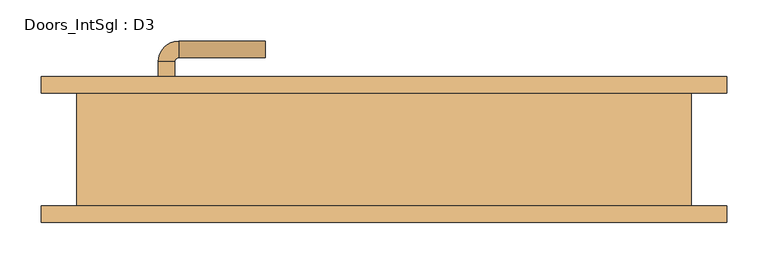
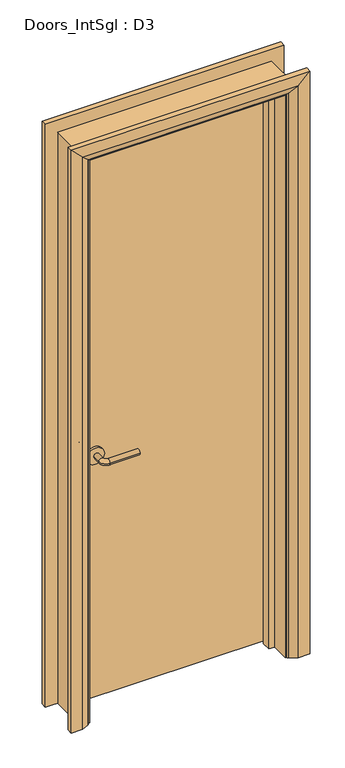
"""IFC4 building model written with IfcOpenShell, lengths in millimetres: door geometry, Doors_IntSgl : D3."""

from ifc_helpers import new_model, si_unit, point, frame, frame_2d, origin, place, context, project, spatial, polyline, circle_curve, ellipse_curve, trimmed, segment, composite_curve, outline, extrude, faceted_brep, source, transform, mapped, element, save
from ifc_brep_helpers import plane_surface, cylinder_surface, revolved_surface, advanced_brep


def doors_intsgl_d3_a434ac6e(model_context):
    return source(origin(), model_context, "Body", "SolidModel", [
        advanced_brep(
        [(-274.0, 22.58, 900.0), (-254.0, 22.58, 900.0), (-254.0, -7.42, 900.0), (-274.0, -7.42, 900.0), (-249.0, -12.42, 900.0), (-249.0, -32.42, 900.0), (-144.0, -32.42, 900.0), (-144.0, -12.42, 900.0)],
        [
            (0, 1, circle_curve(frame((-264.0, 22.58, 900.0), z_axis=(0.0, 1.0, 0.0), x_axis=(1.0, 0.0, 0.0)), 10.0)),
            (1, 0, circle_curve(frame((-264.0, 22.58, 900.0), z_axis=(0.0, 1.0, 0.0), x_axis=(1.0, 0.0, 0.0)), 10.0)),
            (1, 2),
            (2, 3, circle_curve(frame((-264.0, -7.42, 900.0), z_axis=(0.0, 1.0, 0.0), x_axis=(1.0, 0.0, 0.0)), 10.0)),
            (3, 0),
            (3, 2, circle_curve(frame((-264.0, -7.42, 900.0), z_axis=(0.0, 1.0, 0.0), x_axis=(1.0, 0.0, 0.0)), 10.0)),
            (4, 5, circle_curve(frame((-249.0, -22.42, 900.0), z_axis=(-1.0, 0.0, 0.0), x_axis=(0.0, 1.0, 0.0)), 10.0)),
            (5, 3, circle_curve(frame((-249.0, -7.42, 900.0), z_axis=(0.0, 0.0, -1.0), x_axis=(-1.0, 0.0, 0.0)), 25.0)),
            (2, 4, circle_curve(frame((-249.0, -7.42, 900.0), z_axis=(0.0, 0.0, 1.0), x_axis=(-1.0, 0.0, 0.0)), 5.0)),
            (5, 4, circle_curve(frame((-249.0, -22.42, 900.0), z_axis=(-1.0, 0.0, 0.0), x_axis=(0.0, 1.0, 0.0)), 10.0)),
            (6, 7, circle_curve(frame((-144.0, -22.42, 900.0), z_axis=(1.0, 0.0, 0.0), x_axis=(0.0, 1.0, 0.0)), 10.0)),
            (7, 6, circle_curve(frame((-144.0, -22.42, 900.0), z_axis=(1.0, 0.0, 0.0), x_axis=(0.0, 1.0, 0.0)), 10.0)),
            (4, 7),
            (6, 5),
        ],
        [
            plane_surface(frame((-264.0, 22.58, 900.0), z_axis=(0.0, 1.0, 0.0), x_axis=(0.0, 0.0, 1.0))),
            cylinder_surface(frame((-264.0, 22.58, 900.0), z_axis=(0.0, 1.0, 0.0), x_axis=(1.0, 0.0, 0.0)), 10.0),
            revolved_surface(trimmed(ellipse_curve(frame((-264.0, -7.42, 900.0), z_axis=(0.0, -1.0, 0.0), x_axis=(1.0, 0.0, 0.0)), 10.0, 10.0), [point((-274.0, -7.42, 900.0))], [point((-254.0, -7.42, 900.0))], True, "CARTESIAN"), (-249.0, -7.42, 900.0), (0.0, 0.0, -1.0)),
            revolved_surface(trimmed(ellipse_curve(frame((-264.0, -7.42, 900.0), z_axis=(0.0, -1.0, 0.0), x_axis=(1.0, 0.0, 0.0)), 10.0, 10.0), [point((-254.0, -7.42, 900.0))], [point((-274.0, -7.42, 900.0))], True, "CARTESIAN"), (-249.0, -7.42, 900.0), (0.0, 0.0, -1.0)),
            plane_surface(frame((-144.0, -22.42, 900.0), z_axis=(1.0, 0.0, 0.0), x_axis=(0.0, 0.0, 1.0))),
            cylinder_surface(frame((-249.0, -22.42, 900.0), z_axis=(-1.0, 0.0, 0.0), x_axis=(0.0, 1.0, 0.0)), 10.0),
        ],
        [
            (0, [[1, 2]]),
            (1, [[3, 4, 5, -2]]),
            (1, [[-5, 6, -3, -1]]),
            (2, [[7, 8, -4, 9]]),
            (3, [[10, -9, -6, -8]]),
            (4, [[11, 12]]),
            (5, [[13, -11, 14, -7]]),
            (5, [[-14, -12, -13, -10]]),
        ],
    ),
        extrude(outline(composite_curve([segment(trimmed(circle_curve(frame_2d((900.0, -266.5)), 30.0), [point((900.0, -296.5))], [point((900.0, -236.5))], False, "CARTESIAN"), True, "CONTINUOUS"), segment(trimmed(circle_curve(frame_2d((900.0, -266.5)), 30.0), [point((900.0, -236.5))], [point((900.0, -296.5))], False, "CARTESIAN"), True, "CONTINUOUS")], self_intersect=False)), frame((0.0, 22.58, 0.0), z_axis=(0.0, 1.0, 0.0), x_axis=(0.0, 0.0, 1.0)), (0.0, 0.0, 1.0), 8.0),
        advanced_brep(
        [(-274.0, 76.58, 900.0), (-254.0, 76.58, 900.0), (-274.0, 106.58, 900.0), (-254.0, 106.58, 900.0), (-249.0, 111.58, 900.0), (-249.0, 131.58, 900.0), (-144.0, 131.58, 900.0), (-144.0, 111.58, 900.0)],
        [
            (0, 1, circle_curve(frame((-264.0, 76.58, 900.0), z_axis=(0.0, -1.0, 0.0), x_axis=(1.0, 0.0, 0.0)), 10.0)),
            (1, 0, circle_curve(frame((-264.0, 76.58, 900.0), z_axis=(0.0, -1.0, 0.0), x_axis=(1.0, 0.0, 0.0)), 10.0)),
            (0, 2),
            (2, 3, circle_curve(frame((-264.0, 106.58, 900.0), z_axis=(0.0, -1.0, 0.0), x_axis=(1.0, 0.0, 0.0)), 10.0)),
            (3, 1),
            (3, 2, circle_curve(frame((-264.0, 106.58, 900.0), z_axis=(0.0, -1.0, 0.0), x_axis=(1.0, 0.0, 0.0)), 10.0)),
            (4, 3, circle_curve(frame((-249.0, 106.58, 900.0), z_axis=(0.0, 0.0, 1.0), x_axis=(-1.0, 0.0, 0.0)), 5.0)),
            (2, 5, circle_curve(frame((-249.0, 106.58, 900.0), z_axis=(0.0, 0.0, -1.0), x_axis=(-1.0, 0.0, 0.0)), 25.0)),
            (5, 4, circle_curve(frame((-249.0, 121.58, 900.0), z_axis=(-1.0, 0.0, 0.0), x_axis=(0.0, -1.0, 0.0)), 10.0)),
            (4, 5, circle_curve(frame((-249.0, 121.58, 900.0), z_axis=(-1.0, 0.0, 0.0), x_axis=(0.0, -1.0, 0.0)), 10.0)),
            (6, 7, circle_curve(frame((-144.0, 121.58, 900.0), z_axis=(1.0, 0.0, 0.0), x_axis=(0.0, -1.0, 0.0)), 10.0)),
            (7, 6, circle_curve(frame((-144.0, 121.58, 900.0), z_axis=(1.0, 0.0, 0.0), x_axis=(0.0, -1.0, 0.0)), 10.0)),
            (5, 6),
            (7, 4),
        ],
        [
            plane_surface(frame((-264.0, 76.58, 900.0), z_axis=(0.0, -1.0, 0.0), x_axis=(0.0, 0.0, 1.0))),
            cylinder_surface(frame((-264.0, 76.58, 900.0), z_axis=(0.0, -1.0, 0.0), x_axis=(1.0, 0.0, 0.0)), 10.0),
            revolved_surface(trimmed(ellipse_curve(frame((-264.0, 106.58, 900.0), z_axis=(0.0, -1.0, 0.0), x_axis=(1.0, 0.0, 0.0)), 10.0, 10.0), [point((-274.0, 106.58, 900.0))], [point((-254.0, 106.58, 900.0))], True, "CARTESIAN"), (-249.0, 106.58, 900.0), (0.0, 0.0, -1.0)),
            revolved_surface(trimmed(ellipse_curve(frame((-264.0, 106.58, 900.0), z_axis=(0.0, -1.0, 0.0), x_axis=(1.0, 0.0, 0.0)), 10.0, 10.0), [point((-254.0, 106.58, 900.0))], [point((-274.0, 106.58, 900.0))], True, "CARTESIAN"), (-249.0, 106.58, 900.0), (0.0, 0.0, -1.0)),
            plane_surface(frame((-144.0, 121.58, 900.0), z_axis=(1.0, 0.0, 0.0), x_axis=(0.0, 0.0, 1.0))),
            cylinder_surface(frame((-249.0, 121.58, 900.0), z_axis=(-1.0, 0.0, 0.0), x_axis=(0.0, -1.0, 0.0)), 10.0),
        ],
        [
            (0, [[1, 2]]),
            (1, [[-1, 3, 4, 5]]),
            (1, [[-2, -5, 6, -3]]),
            (2, [[7, -4, 8, 9]]),
            (3, [[-8, -6, -7, 10]]),
            (4, [[11, 12]]),
            (5, [[-9, 13, -12, 14]]),
            (5, [[-10, -14, -11, -13]]),
        ],
    ),
        extrude(outline(composite_curve([segment(trimmed(circle_curve(frame_2d((900.0, -266.5)), 30.0), [point((900.0, -296.5))], [point((900.0, -236.5))], False, "CARTESIAN"), True, "CONTINUOUS"), segment(trimmed(circle_curve(frame_2d((900.0, -266.5)), 30.0), [point((900.0, -236.5))], [point((900.0, -296.5))], False, "CARTESIAN"), True, "CONTINUOUS")], self_intersect=False)), frame((0.0, 68.58, 0.0), z_axis=(0.0, 1.0, 0.0), x_axis=(0.0, 0.0, 1.0)), (0.0, 0.0, 1.0), 8.0),
        extrude(outline(polyline([(339.0, 30.58), (-339.0, 30.58), (-339.0, 68.58), (339.0, 68.58), (339.0, 30.58)])), frame((0.0, 0.0, 8.0), z_axis=(0.0, 0.0, 1.0), x_axis=(1.0, 0.0, 0.0)), (0.0, 0.0, 1.0), 2060.0),
        advanced_brep(
        [(416.0, 88.58, 0.0), (416.0, 68.58, 0.0), (346.0, 68.58, 0.0), (350.0, 74.58, 0.0), (376.0, 88.58, 0.0), (416.0, 88.58, 2145.0), (416.0, 68.58, 2145.0), (-416.0, 68.58, 2145.0), (-416.0, 68.58, 0.0), (-346.0, 68.58, 0.0), (-346.0, 68.58, 2075.0), (346.0, 68.58, 2075.0), (350.0, 74.58, 2079.0), (376.0, 88.58, 2105.0), (-376.0, 88.58, 2105.0), (-376.0, 88.58, 0.0), (-416.0, 88.58, 0.0), (-416.0, 88.58, 2145.0), (-350.0, 74.58, 0.0), (-350.0, 74.58, 2079.0)],
        [
            (0, 1),
            (1, 2),
            (2, 3, circle_curve(frame((354.0, 67.58, 0.0), z_axis=(0.0, 0.0, -1.0), x_axis=(1.0, 0.0, 0.0)), 8.0622577)),
            (3, 4),
            (4, 0),
            (0, 5),
            (5, 6),
            (6, 1),
            (6, 7),
            (7, 8),
            (8, 9),
            (9, 10),
            (10, 11),
            (11, 2),
            (11, 12, ellipse_curve(frame((354.0, 67.58, 2083.0), z_axis=(0.7071067811865475, 0.0, -0.7071067811865475), x_axis=(-0.7071067811865474, 0.0, -0.7071067811865476)), 11.4017543, 8.0622577)),
            (12, 3),
            (12, 13),
            (13, 4),
            (13, 14),
            (14, 15),
            (15, 16),
            (16, 17),
            (17, 5),
            (7, 17),
            (16, 8),
            (15, 18),
            (18, 9, circle_curve(frame((-354.0, 67.58, 0.0), z_axis=(0.0, 0.0, -1.0), x_axis=(-1.0, 0.0, 0.0)), 8.0622577)),
            (19, 10, ellipse_curve(frame((-354.0, 67.58, 2083.0), z_axis=(-0.7071067811865475, 0.0, -0.7071067811865475), x_axis=(-0.7071067811865474, 0.0, 0.7071067811865476)), 11.4017543, 8.0622577)),
            (18, 19),
            (14, 19),
            (19, 12),
        ],
        [
            plane_surface(frame((346.0, 68.58, 0.0), z_axis=(0.0, 0.0, -1.0), x_axis=(0.0, -1.0, 0.0))),
            plane_surface(frame((416.0, 88.58, 0.0), z_axis=(1.0, 0.0, 0.0), x_axis=(0.0, 0.0, 1.0))),
            plane_surface(frame((416.0, 68.58, 0.0), z_axis=(0.0, -1.0, 0.0), x_axis=(0.0, 0.0, 1.0))),
            cylinder_surface(frame((354.0, 67.58, 0.0), z_axis=(0.0, 0.0, -1.0), x_axis=(1.0, 0.0, 0.0)), 8.0622577),
            plane_surface(frame((350.0, 74.58, 0.0), z_axis=(-0.4740998230350126, 0.880471099922178, 0.0), x_axis=(0.0, 0.0, 1.0))),
            plane_surface(frame((376.0, 88.58, 0.0), z_axis=(0.0, 1.0, 0.0), x_axis=(0.0, 0.0, 1.0))),
            plane_surface(frame((-416.0, 88.58, 2145.0), z_axis=(-1.0, 0.0, 0.0), x_axis=(0.0, 0.0, -1.0))),
            plane_surface(frame((-346.0, 68.58, 0.0), z_axis=(0.0, 0.0, -1.0), x_axis=(0.0, -1.0, 0.0))),
            cylinder_surface(frame((-354.0, 67.58, 2075.0), z_axis=(0.0, 0.0, 1.0), x_axis=(-1.0, 0.0, 0.0)), 8.0622577),
            plane_surface(frame((-350.0, 74.58, 2079.0), z_axis=(0.47409982303501824, 0.8804710999221749, 0.0), x_axis=(0.0, 0.0, -1.0))),
            plane_surface(frame((416.0, 88.58, 2145.0), z_axis=(0.0, 0.0, 1.0), x_axis=(-1.0, 0.0, 0.0))),
            cylinder_surface(frame((346.0, 67.58, 2083.0), z_axis=(1.0, 0.0, 0.0), x_axis=(0.0, 0.0, 1.0)), 8.0622577),
            plane_surface(frame((350.0, 74.58, 2079.0), z_axis=(0.0, 0.8804710999221764, -0.4740998230350154), x_axis=(-1.0, 0.0, 0.0))),
        ],
        [
            (0, [[1, 2, 3, 4, 5]]),
            (1, [[-1, 6, 7, 8]]),
            (2, [[-2, -8, 9, 10, 11, 12, 13, 14]]),
            (3, [[-3, -14, 15, 16]]),
            (4, [[-4, -16, 17, 18]]),
            (5, [[-5, -18, 19, 20, 21, 22, 23, -6]]),
            (6, [[24, -22, 25, -10]]),
            (7, [[-21, 26, 27, -11, -25]]),
            (8, [[28, -12, -27, 29]]),
            (9, [[30, -29, -26, -20]]),
            (10, [[-7, -23, -24, -9]]),
            (11, [[-15, -13, -28, 31]]),
            (12, [[-17, -31, -30, -19]]),
        ],
    ),
        extrude(outline(polyline([(0.0, -341.0), (0.0, -322.0), (2051.0, -322.0), (2051.0, 322.0), (0.0, 322.0), (0.0, 341.0), (2070.0, 341.0), (2070.0, -341.0), (0.0, -341.0)])), frame((0.0, -3.42, 0.0), z_axis=(0.0, 1.0, 0.0), x_axis=(0.0, 0.0, 1.0)), (0.0, 0.0, 1.0), 32.0),
        advanced_brep(
        [(-416.0, -88.58, 0.0), (-416.0, -68.58, 0.0), (-346.0, -68.58, 0.0), (-350.0, -74.58, 0.0), (-376.0, -88.58, 0.0), (-416.0, -88.58, 2145.0), (-416.0, -68.58, 2145.0), (-346.0, -68.58, 2075.0), (-350.0, -74.58, 2079.0), (-376.0, -88.58, 2105.0), (416.0, -88.58, 0.0), (376.0, -88.58, 0.0), (350.0, -74.58, 0.0), (346.0, -68.58, 0.0), (416.0, -68.58, 0.0), (416.0, -88.58, 2145.0), (376.0, -88.58, 2105.0), (350.0, -74.58, 2079.0), (346.0, -68.58, 2075.0), (416.0, -68.58, 2145.0)],
        [
            (0, 1),
            (1, 2),
            (2, 3, circle_curve(frame((-354.0, -67.58, 0.0), z_axis=(0.0, 0.0, -1.0), x_axis=(-1.0, 0.0, 0.0)), 8.0622577)),
            (3, 4),
            (4, 0),
            (0, 5),
            (5, 6),
            (6, 1),
            (6, 7),
            (7, 2),
            (7, 8, ellipse_curve(frame((-354.0, -67.58, 2083.0), z_axis=(-0.7071067811865475, 0.0, -0.7071067811865475), x_axis=(0.7071067811865474, 0.0, -0.7071067811865476)), 11.4017543, 8.0622577)),
            (8, 3),
            (8, 9),
            (9, 4),
            (9, 5),
            (10, 11),
            (11, 12),
            (12, 13, circle_curve(frame((354.0, -67.58, 0.0), z_axis=(0.0, 0.0, -1.0), x_axis=(1.0, 0.0, 0.0)), 8.0622577)),
            (13, 14),
            (14, 10),
            (15, 16),
            (16, 11),
            (10, 15),
            (16, 17),
            (17, 12),
            (17, 18, ellipse_curve(frame((354.0, -67.58, 2083.0), z_axis=(0.7071067811865475, 0.0, -0.7071067811865475), x_axis=(0.7071067811865474, 0.0, 0.7071067811865476)), 11.4017543, 8.0622577)),
            (18, 13),
            (18, 19),
            (19, 14),
            (19, 15),
            (5, 15),
            (19, 6),
            (18, 7),
            (17, 8),
            (16, 9),
        ],
        [
            plane_surface(frame((-346.0, -141.3810989, 0.0), z_axis=(0.0, 0.0, -1.0), x_axis=(1.0, 0.0, 0.0))),
            plane_surface(frame((-416.0, -88.58, 0.0), z_axis=(-1.0, 0.0, 0.0), x_axis=(0.0, 0.0, 1.0))),
            plane_surface(frame((-416.0, -68.58, 0.0), z_axis=(0.0, 1.0, 0.0), x_axis=(0.0, 0.0, 1.0))),
            cylinder_surface(frame((-354.0, -67.58, 0.0), z_axis=(0.0, 0.0, -1.0), x_axis=(-1.0, 0.0, 0.0)), 8.0622577),
            plane_surface(frame((-350.0, -74.58, 0.0), z_axis=(0.4740998230350183, -0.8804710999221749, 0.0), x_axis=(0.0, 0.0, 1.0))),
            plane_surface(frame((-376.0, -88.58, 0.0), z_axis=(0.0, -1.0, 0.0), x_axis=(0.0, 0.0, 1.0))),
            plane_surface(frame((346.0, -141.3810989, 0.0), z_axis=(0.0, 0.0, -1.0), x_axis=(-1.0, 0.0, 0.0))),
            plane_surface(frame((376.0, -88.58, 2105.0), z_axis=(0.0, -1.0, 0.0), x_axis=(0.0, 0.0, -1.0))),
            plane_surface(frame((350.0, -74.58, 2079.0), z_axis=(-0.4740998230350183, -0.8804710999221749, 0.0), x_axis=(0.0, 0.0, -1.0))),
            cylinder_surface(frame((354.0, -67.58, 2075.0), z_axis=(0.0, 0.0, 1.0), x_axis=(1.0, 0.0, 0.0)), 8.0622577),
            plane_surface(frame((416.0, -68.58, 2145.0), z_axis=(0.0, 1.0, 0.0), x_axis=(0.0, 0.0, -1.0))),
            plane_surface(frame((416.0, -88.58, 2145.0), z_axis=(1.0, 0.0, 0.0), x_axis=(0.0, 0.0, -1.0))),
            plane_surface(frame((-416.0, -88.58, 2145.0), z_axis=(0.0, 0.0, 1.0), x_axis=(1.0, 0.0, 0.0))),
            plane_surface(frame((-416.0, -68.58, 2145.0), z_axis=(0.0, 1.0, 0.0), x_axis=(1.0, 0.0, 0.0))),
            cylinder_surface(frame((-346.0, -67.58, 2083.0), z_axis=(-1.0, 0.0, 0.0), x_axis=(0.0, 0.0, 1.0)), 8.0622577),
            plane_surface(frame((-350.0, -74.58, 2079.0), z_axis=(0.0, -0.8804710999221749, -0.4740998230350183), x_axis=(1.0, 0.0, 0.0))),
            plane_surface(frame((-376.0, -88.58, 2105.0), z_axis=(0.0, -1.0, 0.0), x_axis=(1.0, 0.0, 0.0))),
        ],
        [
            (0, [[1, 2, 3, 4, 5]]),
            (1, [[-1, 6, 7, 8]]),
            (2, [[-2, -8, 9, 10]]),
            (3, [[-3, -10, 11, 12]]),
            (4, [[-4, -12, 13, 14]]),
            (5, [[-5, -14, 15, -6]]),
            (6, [[16, 17, 18, 19, 20]]),
            (7, [[21, 22, -16, 23]]),
            (8, [[24, 25, -17, -22]]),
            (9, [[26, 27, -18, -25]]),
            (10, [[28, 29, -19, -27]]),
            (11, [[30, -23, -20, -29]]),
            (12, [[-7, 31, -30, 32]]),
            (13, [[-9, -32, -28, 33]]),
            (14, [[-11, -33, -26, 34]]),
            (15, [[-13, -34, -24, 35]]),
            (16, [[-15, -35, -21, -31]]),
        ],
    ),
        faceted_brep([(-341.0, 68.58, 0.0), (-341.0, -68.58, 0.0), (-373.0, -68.58, 0.0), (-373.0, 68.58, 0.0), (-341.0, 68.58, 2070.0), (-341.0, -68.58, 2070.0), (-373.0, -68.58, 2102.0), (-373.0, 68.58, 2102.0), (341.0, 68.58, 0.0), (373.0, 68.58, 0.0), (373.0, -68.58, 0.0), (341.0, -68.58, 0.0), (341.0, 68.58, 2070.0), (373.0, 68.58, 2102.0), (373.0, -68.58, 2102.0), (341.0, -68.58, 2070.0)], [[[0, 1, 2, 3]], [[1, 0, 4, 5]], [[2, 1, 5, 6]], [[3, 2, 6, 7]], [[0, 3, 7, 4]], [[8, 9, 10, 11]], [[12, 13, 9, 8]], [[13, 14, 10, 9]], [[14, 15, 11, 10]], [[15, 12, 8, 11]], [[5, 4, 12, 15]], [[6, 5, 15, 14]], [[7, 6, 14, 13]], [[4, 7, 13, 12]]]),
    ])


if __name__ == "__main__":
    model = new_model("IFC4")
    model_context = context("Model", 3, world=origin())
    ifc_project = project(units=[si_unit("LENGTHUNIT", "METRE", prefix="MILLI")], contexts=[model_context])
    site = spatial("IfcSite", under=ifc_project)
    building = spatial("IfcBuilding", under=site)
    placement = place(None, origin())
    doors_intsgl_d3_shape = doors_intsgl_d3_a434ac6e(model_context)
    element("IfcDoor", 1, ObjectType="Doors_IntSgl : D3", at=placement, inside=building, context=model_context, shape_type="MappedRepresentation", body=[
        mapped(doors_intsgl_d3_shape, transform((0.0, 0.0, 0.0), x_axis=(1.0, 0.0, 0.0), y_axis=(0.0, 1.0, 0.0), z_axis=(0.0, 0.0, 1.0))),
    ])
    save(model, "model.ifc")

# Revit data of these elements
# Type "Doors_IntSgl : D3"
#   Type Mark = "48"
#   Type Comments = "Internal Single"
#   Operation = "SingleSwingRight"
#   Manufacturer = "Revit"
#   Keynote = "L20"
#   Description = "Internal Single Door"
#   Analytic Construction = "Metal"
#   UnderCut = 8 mm
#   Tolerance = 2 mm
#   Thickness = 38 mm
#   Thermal Resistance (R) = 0.270117 (m²·K)/W
#   Structural Tolerance = 8 mm
#   StopDepth = 32 mm
#   Stop Thickness = 19 mm
#   Rough Width = 762 mm
#   Rough Height = 2110 mm
#   Height to Top Lock Rail = 1000 mm
#   Heat Transfer Coefficient (U) = 3.7021 W/(m²·K)
#   Handle Z Distance = 900 mm
#   Handle X Distance = 75 mm
#   Frame Thickness = 32 mm
#   Door Panel Width = 678 mm
#   Door Panel Thickness = 38 mm
#   Door Panel Offset = 0 mm
#   Height = 2110 mm
#   Width = 762 mm
#   Door Panel Height = 2060 mm
#   Architrave Setback = 5 mm
#   Vis - Ironmongery = yes
#   Material Ironmongery = Door - Handle
#   Material Frame = Door - Frame/Mullion (1)
#   Material Door = Door - Panel
#   Material Architrave = Door - Architrave
#   Visual Light Transmittance = 0
#   Solar Heat Gain Coefficient = 0
#   Function = (empty or 0)
#   Wall Closure = (empty or 0)
# Element 1 (IfcDoor, "Doors_IntSgl : D3")
#   Materials on its faces: "Door - Architrave", "Door - Handle", "Door - Frame/Mullion (1)", "Door - Panel"
# Materials
#   "Door - Handle": colour RGB 0 0 0, transparency 0, Keynote = "P21", Cost = 0
#   "Door - Frame/Mullion (1)": class "Wood", colour RGB 212 179 113, transparency 0, Keynote = "L20", Cost = 0
#   "Door - Panel": class "Wood", colour RGB 210 159 95, transparency 0, Keynote = "L20", Cost = 0
#   "Door - Architrave": class "Wood", colour RGB 154 90 5, transparency 0, Keynote = "P20", Cost = 0
